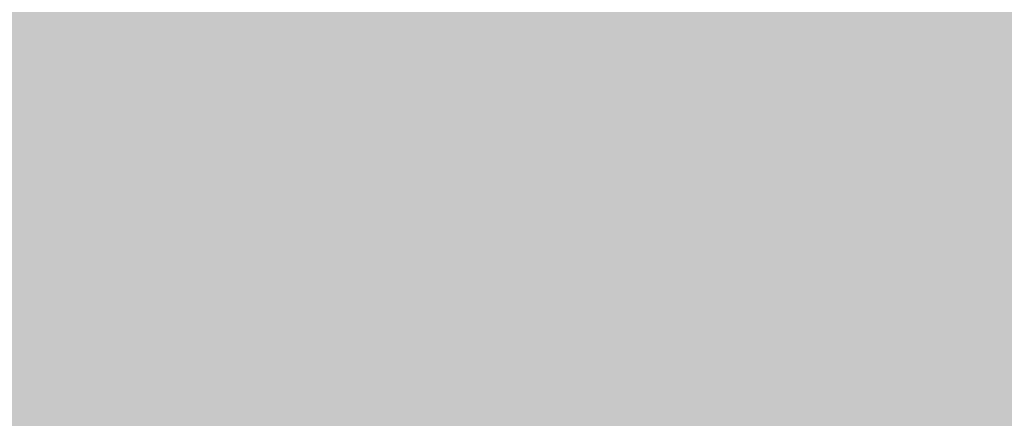
# Model space of a CAD drawing. Units: millimetres. Extents: x 0 to 2267, y 0 to 1823.
# Tile 102 of 256: x 1600.369 to 1605.705, y 1228.277 to 1230.439. Entities that reach past the tile are written whole.
import ezdxf

# ---------------------------------------------------------------- set-up
doc = ezdxf.new("R2010")
doc.units = ezdxf.units.MM
doc.header["$MEASUREMENT"] = 0
doc.layers.add('M-HATC', color=252, linetype='Continuous', lineweight=18)

msp = doc.modelspace()

# ---------------------------------------------------------------- hatches: boundary and pattern name
at = {"layer": 'M-HATC'}
h = msp.add_hatch(color=256, dxfattribs=at)
h.dxf.hatch_style = 1
h.paths.add_polyline_path([(2055.771, 1603.062), (1381.0868, 1603.062), (1381.0868, 1598.062), (2055.771, 1598.062)])
h.paths.add_polyline_path([(2055.771, 1598.062), (1381.0868, 1598.062), (1381.0868, 1593.062), (2055.771, 1593.062)])
h.paths.add_polyline_path([(2051.3074, 1536.7609), (1385.5504, 1536.7609), (1385.5504, 1526.7609), (1387.5504, 1526.7609), (1388.5366, 1525.0528), (1385.3319, 1521.2335), (1385.3319, 1521.2226), (2050.2542, 1522.7491), (2048.3212, 1525.0528), (2049.3074, 1526.7609), (2051.3074, 1526.7609)])
edge = h.paths.add_edge_path()
edge.add_arc((1847.5345, 1379.1492), 135, 222.603061, 222.890851, ccw=False)
edge.add_line((1748.1663, 1287.7656), (1683.0921, 1287.7656))
edge.add_arc((1583.7239, 1379.1492), 135, 317.109149, 317.396939, ccw=False)
edge.add_arc((1678.9686, 1290.6707), 5, 222.8909, 317.1091, ccw=False)
edge.add_arc((1774.2133, 1379.1492), 135, 222.603061, 222.890851, ccw=False)
edge.add_line((1674.8451, 1287.7656), (1609.7709, 1287.7656))
edge.add_arc((1510.4027, 1379.1492), 135, 317.109149, 317.396939, ccw=False)
edge.add_arc((1605.6474, 1290.6707), 5, 222.8909, 317.1091, ccw=False)
edge.add_arc((1700.8921, 1379.1492), 135, 222.603061, 222.890851, ccw=False)
edge.add_line((1601.5239, 1287.7656), (1536.4497, 1287.7656))
edge.add_arc((1437.0815, 1379.1492), 135, 317.109149, 317.396939, ccw=False)
edge.add_arc((1532.3262, 1290.6707), 5, 222.8909, 317.1091, ccw=False)
edge.add_arc((1627.5709, 1379.1492), 135, 222.603061, 222.890851, ccw=False)
edge.add_line((1528.2027, 1287.7656), (1505.9289, 1287.7656))
edge.add_spline(control_points=[(1505.9289, 1287.7656), (1504.2622, 1287.7656), (1504.2622, 1282.7656), (1505.9289, 1282.7656)], knot_values=[0, 0, 0, 0, 5, 5, 5, 5], degree=3, periodic=0)
edge.add_line((1505.9289, 1282.7656), (1930.9289, 1282.7656))
edge.add_spline(control_points=[(1930.9289, 1282.7656), (1932.5956, 1282.7656), (1932.5956, 1287.7656), (1930.9289, 1287.7656)], knot_values=[0, 0, 0, 0, 5, 5, 5, 5], degree=3, periodic=0)
edge.add_line((1930.9289, 1287.7656), (1903.0557, 1287.7656))
edge.add_arc((1803.6875, 1379.1492), 135, 317.109149, 317.396939, ccw=False)
edge.add_arc((1898.9322, 1290.6707), 5, 222.8909, 317.1091, ccw=False)
edge.add_arc((1994.1769, 1379.1492), 135, 222.603061, 222.890851, ccw=False)
edge.add_line((1894.8087, 1287.7656), (1829.7345, 1287.7656))
edge.add_arc((1730.3663, 1379.1492), 135, 317.109149, 317.396939, ccw=False)
edge.add_arc((1825.611, 1290.6707), 5, 222.8909, 317.1091, ccw=False)
edge.add_arc((1920.8557, 1379.1492), 135, 222.603061, 222.890851, ccw=False)
edge.add_line((1821.4875, 1287.7656), (1756.4133, 1287.7656))
edge.add_arc((1657.0451, 1379.1492), 135, 317.109149, 317.396939, ccw=False)
edge.add_arc((1752.2898, 1290.6707), 5, 222.8909, 317.1091, ccw=False)
edge = h.paths.add_edge_path()
edge.add_spline(control_points=[(1843.4289, 1227.2475), (1845.0956, 1227.2475), (1845.0956, 1232.2475), (1843.4289, 1232.2475)], knot_values=[0, 0, 0, 0, 5, 5, 5, 5], degree=3, periodic=0)
edge.add_line((1843.4289, 1232.2475), (1593.4289, 1232.2475))
edge.add_spline(control_points=[(1593.4289, 1232.2475), (1591.7622, 1232.2475), (1591.7622, 1227.2475), (1593.4289, 1227.2475)], knot_values=[0, 0, 0, 0, 5, 5, 5, 5], degree=3, periodic=0)
edge.add_line((1593.4289, 1227.2475), (1843.4289, 1227.2475))
h.paths.add_polyline_path([(1905.9289, 1127.4171), (1530.9289, 1127.4171, 0.414214), (1520.9289, 1117.4171), (1530.9289, 1117.4171), (1915.9289, 1117.4171, 0.414214)])
edge = h.paths.add_edge_path()
edge.add_arc((1397.0858, 1498.4078), 12.7299, 90.78215, 190.87871, ccw=False)
edge.add_line((1396.912, 1511.1365), (1428.0097, 1511.3488))
edge.add_line((1428.0097, 1511.3488), (1433.0097, 1511.3488))
edge.add_line((1433.0097, 1511.3488), (1434.439, 1511.3488))
edge.add_arc((1419.474, 1498.0804), 20, 41.561, 74.08211)
edge.add_line((1424.9592, 1517.3135), (1399.9351, 1517.2561))
edge.add_spline(control_points=[(1399.9307, 1517.2561), (1399.884, 1517.2131), (1399.8328, 1517.1689), (1399.7774, 1517.1236)], knot_values=[11.567499, 11.567499, 11.567499, 11.567499, 11.814249, 11.814249, 11.814249, 11.814249], degree=3, periodic=0)
edge.add_spline(control_points=[(1399.6328, 1517.0099), (1399.5831, 1516.9721), (1399.5307, 1516.9338), (1399.4759, 1516.8947)], knot_values=[11.167718, 11.167718, 11.167718, 11.167718, 11.365188, 11.365188, 11.365188, 11.365188], degree=3, periodic=0)
edge.add_spline(control_points=[(1399.3398, 1516.8001), (1399.1514, 1516.6719), (1398.9384, 1516.5377), (1398.704, 1516.3994)], knot_values=[10.376405, 10.376405, 10.376405, 10.376405, 11.00994, 11.00994, 11.00994, 11.00994], degree=3, periodic=0)
edge.add_spline(control_points=[(1398.6572, 1516.3719), (1398.5789, 1516.326), (1398.4983, 1516.2797), (1398.4155, 1516.2331)], knot_values=[10.125175, 10.125175, 10.125175, 10.125175, 10.334406, 10.334406, 10.334406, 10.334406], degree=3, periodic=0)
edge.add_spline(control_points=[(1398.2642, 1516.1487), (1398.196, 1516.1111), (1398.1263, 1516.0732), (1398.0555, 1516.0351)], knot_values=[9.832246, 9.832246, 9.832246, 9.832246, 9.999658, 9.999658, 9.999658, 9.999658], degree=3, periodic=0)
edge.add_spline(control_points=[(1397.9987, 1516.0048), (1397.7312, 1515.8621), (1397.446, 1515.7171), (1397.1466, 1515.5714)], knot_values=[9.161808, 9.161808, 9.161808, 9.161808, 9.787769, 9.787769, 9.787769, 9.787769], degree=3, periodic=0)
edge.add_spline(control_points=[(1397.1466, 1515.5714), (1396.8418, 1515.423), (1396.5222, 1515.274), (1396.1914, 1515.1262)], knot_values=[8.524455, 8.524455, 8.524455, 8.524455, 9.161808, 9.161808, 9.161808, 9.161808], degree=3, periodic=0)
edge.add_spline(control_points=[(1396.0777, 1515.0756), (1395.9854, 1515.0348), (1395.8922, 1514.994), (1395.7983, 1514.9534)], knot_values=[8.275193, 8.275193, 8.275193, 8.275193, 8.451726, 8.451726, 8.451726, 8.451726], degree=3, periodic=0)
edge.add_spline(control_points=[(1395.6018, 1514.8691), (1395.4997, 1514.8257), (1395.3968, 1514.7824), (1395.2932, 1514.7394)], knot_values=[7.962917, 7.962917, 7.962917, 7.962917, 8.152764, 8.152764, 8.152764, 8.152764], degree=3, periodic=0)
edge.add_spline(control_points=[(1395.2116, 1514.7057), (1394.8278, 1514.5475), (1394.4345, 1514.3929), (1394.0364, 1514.2442)], knot_values=[7.21254, 7.21254, 7.21254, 7.21254, 7.913148, 7.913148, 7.913148, 7.913148], degree=3, periodic=0)
edge.add_spline(control_points=[(1394.0364, 1514.2442), (1393.7076, 1514.1214), (1393.3754, 1514.0027), (1393.0427, 1513.8895)], knot_values=[6.633733, 6.633733, 6.633733, 6.633733, 7.21254, 7.21254, 7.21254, 7.21254], degree=3, periodic=0)
edge.add_spline(control_points=[(1392.8214, 1513.815), (1392.7198, 1513.7812), (1392.6181, 1513.7479), (1392.5166, 1513.7152)], knot_values=[6.328796, 6.328796, 6.328796, 6.328796, 6.505493, 6.505493, 6.505493, 6.505493], degree=3, periodic=0)
edge.add_spline(control_points=[(1392.5166, 1513.7152), (1392.3187, 1513.6515), (1392.1212, 1513.59), (1391.9244, 1513.531)], knot_values=[5.984605, 5.984605, 5.984605, 5.984605, 6.328796, 6.328796, 6.328796, 6.328796], degree=3, periodic=0)
edge.add_spline(control_points=[(1391.7915, 1513.4915), (1391.3122, 1513.3501), (1390.8384, 1513.2239), (1390.3784, 1513.1171)], knot_values=[5.066697, 5.066697, 5.066697, 5.066697, 5.907055, 5.907055, 5.907055, 5.907055], degree=3, periodic=0)
edge.add_spline(control_points=[(1390.3784, 1513.1171), (1390.1797, 1513.071), (1389.9836, 1513.0284), (1389.7907, 1512.9899)], knot_values=[4.70367, 4.70367, 4.70367, 4.70367, 5.066695, 5.066695, 5.066695, 5.066695], degree=3, periodic=0)
edge.add_spline(control_points=[(1389.422, 1512.9204), (1389.2459, 1512.8892), (1389.0729, 1512.8617), (1388.9036, 1512.8381)], knot_values=[4.130571, 4.130571, 4.130571, 4.130571, 4.469816, 4.469816, 4.469816, 4.469816], degree=3, periodic=0)
edge.add_spline(control_points=[(1388.9036, 1512.8381), (1388.591, 1512.7946), (1388.2911, 1512.7644), (1388.0071, 1512.7494)], knot_values=[3.504031, 3.504031, 3.504031, 3.504031, 4.130571, 4.130571, 4.130571, 4.130571], degree=3, periodic=0)
edge.add_spline(control_points=[(1387.9356, 1512.7459), (1387.8538, 1512.7423), (1387.7733, 1512.74), (1387.6944, 1512.739)], knot_values=[3.268866, 3.268866, 3.268866, 3.268866, 3.451164, 3.451164, 3.451164, 3.451164], degree=3, periodic=0)
edge.add_spline(control_points=[(1387.3351, 1512.7443), (1387.2076, 1512.7499), (1387.0847, 1512.7597), (1386.967, 1512.7739)], knot_values=[2.670686, 2.670686, 2.670686, 2.670686, 2.984, 2.984, 2.984, 2.984], degree=3, periodic=0)
edge.add_spline(control_points=[(1386.8327, 1512.7922), (1386.8209, 1512.7941), (1386.8092, 1512.7959), (1386.7975, 1512.7979)], knot_values=[2.516981, 2.516981, 2.516981, 2.516981, 2.549528, 2.549528, 2.549528, 2.549528], degree=3, periodic=0)
edge.add_spline(control_points=[(1386.4526, 1512.8735), (1386.4257, 1512.881), (1386.3993, 1512.889), (1386.3733, 1512.8972)], knot_values=[2.095869, 2.095869, 2.095869, 2.095869, 2.17941, 2.17941, 2.17941, 2.17941], degree=3, periodic=0)
edge.add_spline(control_points=[(1386.0691, 1513.0189), (1386.0634, 1513.0217), (1386.0577, 1513.0246), (1386.052, 1513.0275)], knot_values=[1.72453, 1.72453, 1.72453, 1.72453, 1.745933, 1.745933, 1.745933, 1.745933], degree=3, periodic=0)
edge.add_arc((1399.474, 1498.0804), 20, 131.82432, 180)
edge.add_arc((1630.3336, 1505.5484), 250.9708, 181.705176, 236.427975)
edge.add_arc((1605.3399, 1483.3044), 218.7822, 238.660829, 243.34961)
edge.add_arc((1647.0911, 1510.3592), 262.8986, 183.129836, 237.853442, ccw=False)
h.paths.add_polyline_path([(1406.5369, 1391.9644, 0.149382), (1491.5506, 1296.4418, -0.129517)], flags=17)
edge = h.paths.add_edge_path()
edge.add_arc((2037.3838, 1498.0804), 20, 0, 48.26587)
edge.add_spline(control_points=[(2050.6973, 1513.0052), (2050.6512, 1512.9847), (2050.6034, 1512.9655), (2050.5539, 1512.9477)], knot_values=[1.835652, 1.835652, 1.835652, 1.835652, 2.000781, 2.000781, 2.000781, 2.000781], degree=3, periodic=0)
edge.add_spline(control_points=[(2050.4616, 1512.9166), (2050.479, 1512.9221), (2050.4963, 1512.9277), (2050.5133, 1512.9335)], knot_values=[2.045477, 2.045477, 2.045477, 2.045477, 2.101389, 2.101389, 2.101389, 2.101389], degree=3, periodic=0)
edge.add_spline(control_points=[(2050.129, 1512.8342), (2050.1984, 1512.8473), (2050.2657, 1512.8623), (2050.3308, 1512.8792)], knot_values=[2.237629, 2.237629, 2.237629, 2.237629, 2.435841, 2.435841, 2.435841, 2.435841], degree=3, periodic=0)
edge.add_spline(control_points=[(2050.0946, 1512.8278), (2050.1061, 1512.8299), (2050.1176, 1512.832), (2050.129, 1512.8342)], knot_values=[2.435841, 2.435841, 2.435841, 2.435841, 2.468321, 2.468321, 2.468321, 2.468321], degree=3, periodic=0)
edge.add_spline(control_points=[(2049.7843, 1512.7851), (2049.8552, 1512.7922), (2049.9243, 1512.8008), (2049.9917, 1512.8109)], knot_values=[2.563852, 2.563852, 2.563852, 2.563852, 2.748541, 2.748541, 2.748541, 2.748541], degree=3, periodic=0)
edge.add_spline(control_points=[(2049.4052, 1512.7617), (2049.5364, 1512.7653), (2049.6629, 1512.773), (2049.7843, 1512.7851)], knot_values=[2.748541, 2.748541, 2.748541, 2.748541, 3.064882, 3.064882, 3.064882, 3.064882], degree=3, periodic=0)
edge.add_spline(control_points=[(2049.1698, 1512.7597), (2049.2336, 1512.7591), (2049.2965, 1512.7594), (2049.3584, 1512.7606)], knot_values=[3.102309, 3.102309, 3.102309, 3.102309, 3.2503, 3.2503, 3.2503, 3.2503], degree=3, periodic=0)
edge.add_spline(control_points=[(2048.8573, 1512.7691), (2048.9638, 1512.7638), (2049.068, 1512.7606), (2049.1698, 1512.7597)], knot_values=[3.2503, 3.2503, 3.2503, 3.2503, 3.486069, 3.486069, 3.486069, 3.486069], degree=3, periodic=0)
edge.add_spline(control_points=[(2048.6924, 1512.7789), (2048.3729, 1512.8009), (2048.0345, 1512.8411), (2047.6817, 1512.897)], knot_values=[3.606429, 3.606429, 3.606429, 3.606429, 4.2989, 4.2989, 4.2989, 4.2989], degree=3, periodic=0)
edge.add_spline(control_points=[(2047.6817, 1512.897), (2047.5458, 1512.9185), (2047.4077, 1512.9424), (2047.2678, 1512.9685)], knot_values=[4.2989, 4.2989, 4.2989, 4.2989, 4.565769, 4.565769, 4.565769, 4.565769], degree=3, periodic=0)
edge.add_spline(control_points=[(2047.2678, 1512.9685), (2047.1449, 1512.9914), (2047.0207, 1513.016), (2046.8951, 1513.0422)], knot_values=[4.565769, 4.565769, 4.565769, 4.565769, 4.799971, 4.799971, 4.799971, 4.799971], degree=3, periodic=0)
edge.add_spline(control_points=[(2046.8951, 1513.0422), (2046.5286, 1513.1188), (2046.1513, 1513.209), (2045.7676, 1513.3107)], knot_values=[4.799971, 4.799971, 4.799971, 4.799971, 5.483718, 5.483718, 5.483718, 5.483718], degree=3, periodic=0)
edge.add_spline(control_points=[(2045.7676, 1513.3107), (2045.3724, 1513.4154), (2044.9704, 1513.5322), (2044.5662, 1513.6588)], knot_values=[5.483718, 5.483718, 5.483718, 5.483718, 6.187866, 6.187866, 6.187866, 6.187866], degree=3, periodic=0)
edge.add_spline(control_points=[(2044.5662, 1513.6588), (2044.4149, 1513.7061), (2044.2633, 1513.7549), (2044.1116, 1513.8048)], knot_values=[6.187866, 6.187866, 6.187866, 6.187866, 6.451551, 6.451551, 6.451551, 6.451551], degree=3, periodic=0)
edge.add_spline(control_points=[(2044.1116, 1513.8048), (2043.9967, 1513.8427), (2043.8817, 1513.8813), (2043.7668, 1513.9205)], knot_values=[6.451551, 6.451551, 6.451551, 6.451551, 6.651434, 6.651434, 6.651434, 6.651434], degree=3, periodic=0)
edge.add_spline(control_points=[(2043.7668, 1513.9205), (2043.3716, 1514.0554), (2042.9774, 1514.1979), (2042.5886, 1514.3458)], knot_values=[6.651434, 6.651434, 6.651434, 6.651434, 7.338879, 7.338879, 7.338879, 7.338879], degree=3, periodic=0)
edge.add_spline(control_points=[(2042.5886, 1514.3458), (2042.1643, 1514.5071), (2041.7465, 1514.6749), (2041.3409, 1514.846)], knot_values=[7.338879, 7.338879, 7.338879, 7.338879, 8.089209, 8.089209, 8.089209, 8.089209], degree=3, periodic=0)
edge.add_spline(control_points=[(2041.3409, 1514.846), (2041.1028, 1514.9465), (2040.869, 1515.0481), (2040.6405, 1515.1502)], knot_values=[8.089209, 8.089209, 8.089209, 8.089209, 8.529587, 8.529587, 8.529587, 8.529587], degree=3, periodic=0)
edge.add_spline(control_points=[(2040.51, 1515.2089), (2040.0824, 1515.4022), (2039.6747, 1515.5971), (2039.295, 1515.7894)], knot_values=[8.613818, 8.613818, 8.613818, 8.613818, 9.44571, 9.44571, 9.44571, 9.44571], degree=3, periodic=0)
edge.add_spline(control_points=[(2039.295, 1515.7894), (2039.0618, 1515.9075), (2038.8391, 1516.0246), (2038.6288, 1516.1398)], knot_values=[9.44571, 9.44571, 9.44571, 9.44571, 9.956404, 9.956404, 9.956404, 9.956404], degree=3, periodic=0)
edge.add_spline(control_points=[(2038.6288, 1516.1398), (2038.5187, 1516.2001), (2038.4121, 1516.2598), (2038.309, 1516.3189)], knot_values=[9.956404, 9.956404, 9.956404, 9.956404, 10.223542, 10.223542, 10.223542, 10.223542], degree=3, periodic=0)
edge.add_spline(control_points=[(2038.309, 1516.3189), (2038.2138, 1516.3735), (2038.1216, 1516.4276), (2038.0328, 1516.481)], knot_values=[10.223542, 10.223542, 10.223542, 10.223542, 10.47051, 10.47051, 10.47051, 10.47051], degree=3, periodic=0)
edge.add_spline(control_points=[(2038.0328, 1516.481), (2037.7855, 1516.6296), (2037.5639, 1516.773), (2037.3722, 1516.909)], knot_values=[10.47051, 10.47051, 10.47051, 10.47051, 11.15767, 11.15767, 11.15767, 11.15767], degree=3, periodic=0)
edge.add_spline(control_points=[(2037.3722, 1516.909), (2037.2789, 1516.9752), (2037.1927, 1517.0396), (2037.1142, 1517.102)], knot_values=[11.15767, 11.15767, 11.15767, 11.15767, 11.49227, 11.49227, 11.49227, 11.49227], degree=3, periodic=0)
edge.add_spline(control_points=[(2036.8564, 1517.3259), (2036.9148, 1517.2692), (2036.9814, 1517.2103), (2037.0557, 1517.1492)], knot_values=[11.577341, 11.577341, 11.577341, 11.577341, 11.91035, 11.91035, 11.91035, 11.91035], degree=3, periodic=0)
edge.add_spline(control_points=[(2036.8074, 1517.3748), (2036.823, 1517.3587), (2036.8393, 1517.3424), (2036.8564, 1517.3259)], knot_values=[11.91035, 11.91035, 11.91035, 11.91035, 12.007402, 12.007402, 12.007402, 12.007402], degree=3, periodic=0)
edge.add_spline(control_points=[(2036.7017, 1517.494), (2036.7104, 1517.483), (2036.7196, 1517.4719), (2036.7291, 1517.4606)], knot_values=[12.184155, 12.184155, 12.184155, 12.184155, 12.255409, 12.255409, 12.255409, 12.255409], degree=3, periodic=0)
edge.add_spline(control_points=[(2036.6159, 1517.6205), (2036.62, 1517.613), (2036.6243, 1517.6055), (2036.6289, 1517.5979)], knot_values=[12.487913, 12.487913, 12.487913, 12.487913, 12.541035, 12.541035, 12.541035, 12.541035], degree=3, periodic=0)
edge.add_spline(control_points=[(2036.5635, 1517.786), (2036.5637, 1517.7794), (2036.5642, 1517.7726), (2036.565, 1517.7658)], knot_values=[12.911761, 12.911761, 12.911761, 12.911761, 12.968286, 12.968286, 12.968286, 12.968286], degree=3, periodic=0)
edge.add_spline(control_points=[(2036.6166, 1517.9304), (2036.6125, 1517.9259), (2036.6086, 1517.9212), (2036.6049, 1517.9165)], knot_values=[13.382527, 13.382527, 13.382527, 13.382527, 13.433791, 13.433791, 13.433791, 13.433791], degree=3, periodic=0)
edge.add_spline(control_points=[(2036.749, 1518.017), (2036.7361, 1518.0116), (2036.7239, 1518.006), (2036.7124, 1518.0002)], knot_values=[13.726299, 13.726299, 13.726299, 13.726299, 13.809928, 13.809928, 13.809928, 13.809928], degree=3, periodic=0)
edge.add_spline(control_points=[(2036.8604, 1518.0528), (2036.8386, 1518.0474), (2036.8181, 1518.0416), (2036.7988, 1518.0353)], knot_values=[13.910887, 13.910887, 13.910887, 13.910887, 14.02153, 14.02153, 14.02153, 14.02153], degree=3, periodic=0)
edge.add_line((2036.9639, 1518.0804), (2032.3838, 1518.0804))
edge.add_line((2032.3838, 1518.0804), (2027.3838, 1518.0804))
edge.add_line((2027.3838, 1518.0804), (2022.3838, 1518.0804))
edge.add_line((2022.3838, 1518.0804), (2017.3838, 1518.0804))
edge.add_arc((2017.3838, 1498.0804), 20, 90, 138.439)
edge.add_line((2002.4188, 1511.3488), (2003.8481, 1511.3488))
edge.add_line((2003.8481, 1511.3488), (2008.8481, 1511.3488))
edge.add_line((2008.8481, 1511.3488), (2039.772, 1511.1377))
edge.add_arc((2039.772, 1498.4078), 12.7299, -10.87871, 90, ccw=False)
edge.add_arc((1789.7668, 1510.3592), 262.8986, 302.146558, 356.870164, ccw=False)
edge.add_arc((1831.5179, 1483.3044), 218.7822, 296.65039, 301.339171)
edge.add_arc((1806.5242, 1505.5484), 250.9708, 303.572025, 358.294824)
h.paths.add_polyline_path([(2030.321, 1391.9644, -0.129517), (1945.3072, 1296.4418, 0.149382)], flags=17)
edge = h.paths.add_edge_path()
edge.add_spline(control_points=[(2037.2464, 1518.0821), (2037.2898, 1518.081), (2037.3355, 1518.0804), (2037.3838, 1518.0804)], knot_values=[0.000012, 0.000012, 0.000012, 0.000012, 0.144754, 0.144754, 0.144754, 0.144754], degree=3, periodic=0)
edge.add_line((2037.3357, 1518.0804), (2037.0096, 1518.0804))
edge.add_spline(control_points=[(2037.0096, 1518.0804), (2036.9822, 1518.0768), (2036.956, 1518.0727), (2036.9312, 1518.0681)], knot_values=[14.13465, 14.13465, 14.13465, 14.13465, 14.247197, 14.247197, 14.247197, 14.247197], degree=3, periodic=0)
edge.add_spline(control_points=[(2036.9312, 1518.0681), (2036.9276, 1518.0674), (2036.9241, 1518.0667), (2036.9205, 1518.0661)], knot_values=[14.118315, 14.118315, 14.118315, 14.118315, 14.13465, 14.13465, 14.13465, 14.13465], degree=3, periodic=0)
edge.add_spline(control_points=[(2036.9205, 1518.0661), (2036.9118, 1518.0644), (2036.9032, 1518.0626), (2036.8948, 1518.0608)], knot_values=[14.078086, 14.078086, 14.078086, 14.078086, 14.118315, 14.118315, 14.118315, 14.118315], degree=3, periodic=0)
edge.add_spline(control_points=[(2036.8948, 1518.0608), (2036.883, 1518.0583), (2036.8716, 1518.0556), (2036.8604, 1518.0528)], knot_values=[14.02153, 14.02153, 14.02153, 14.02153, 14.078086, 14.078086, 14.078086, 14.078086], degree=3, periodic=0)
edge.add_spline(control_points=[(2036.8604, 1518.0528), (2036.8386, 1518.0474), (2036.8181, 1518.0416), (2036.7988, 1518.0353)], knot_values=[13.910887, 13.910887, 13.910887, 13.910887, 14.02153, 14.02153, 14.02153, 14.02153], degree=3, periodic=0)
edge.add_spline(control_points=[(2036.7988, 1518.0353), (2036.7981, 1518.035), (2036.7974, 1518.0348), (2036.7967, 1518.0346)], knot_values=[13.906906, 13.906906, 13.906906, 13.906906, 13.910887, 13.910887, 13.910887, 13.910887], degree=3, periodic=0)
edge.add_spline(control_points=[(2036.7967, 1518.0346), (2036.7882, 1518.0318), (2036.7799, 1518.0289), (2036.7719, 1518.0259)], knot_values=[13.857826, 13.857826, 13.857826, 13.857826, 13.906906, 13.906906, 13.906906, 13.906906], degree=3, periodic=0)
edge.add_spline(control_points=[(2036.7719, 1518.0259), (2036.764, 1518.023), (2036.7564, 1518.02), (2036.749, 1518.017)], knot_values=[13.809928, 13.809928, 13.809928, 13.809928, 13.857826, 13.857826, 13.857826, 13.857826], degree=3, periodic=0)
edge.add_spline(control_points=[(2036.749, 1518.017), (2036.7361, 1518.0116), (2036.7239, 1518.006), (2036.7124, 1518.0002)], knot_values=[13.726299, 13.726299, 13.726299, 13.726299, 13.809928, 13.809928, 13.809928, 13.809928], degree=3, periodic=0)
edge.add_spline(control_points=[(2036.7124, 1518.0002), (2036.7121, 1518), (2036.7118, 1517.9999), (2036.7115, 1517.9997)], knot_values=[13.723993, 13.723993, 13.723993, 13.723993, 13.726299, 13.726299, 13.726299, 13.726299], degree=3, periodic=0)
edge.add_spline(control_points=[(2036.7115, 1517.9997), (2036.7063, 1517.9971), (2036.7013, 1517.9944), (2036.6965, 1517.9917)], knot_values=[13.686536, 13.686536, 13.686536, 13.686536, 13.723993, 13.723993, 13.723993, 13.723993], degree=3, periodic=0)
edge.add_spline(control_points=[(2036.6965, 1517.9917), (2036.6919, 1517.9891), (2036.6874, 1517.9865), (2036.6831, 1517.9839)], knot_values=[13.651251, 13.651251, 13.651251, 13.651251, 13.686536, 13.686536, 13.686536, 13.686536], degree=3, periodic=0)
edge.add_spline(control_points=[(2036.6831, 1517.9839), (2036.6764, 1517.9798), (2036.67, 1517.9757), (2036.6639, 1517.9714)], knot_values=[13.596804, 13.596804, 13.596804, 13.596804, 13.651251, 13.651251, 13.651251, 13.651251], degree=3, periodic=0)
edge.add_spline(control_points=[(2036.6639, 1517.9714), (2036.6636, 1517.9712), (2036.6633, 1517.9709), (2036.6629, 1517.9707)], knot_values=[13.593956, 13.593956, 13.593956, 13.593956, 13.596804, 13.596804, 13.596804, 13.596804], degree=3, periodic=0)
edge.add_spline(control_points=[(2036.6629, 1517.9707), (2036.6603, 1517.9689), (2036.6577, 1517.967), (2036.6552, 1517.9651)], knot_values=[13.570322, 13.570322, 13.570322, 13.570322, 13.593956, 13.593956, 13.593956, 13.593956], degree=3, periodic=0)
edge.add_spline(control_points=[(2036.6552, 1517.9651), (2036.6525, 1517.9631), (2036.6499, 1517.9611), (2036.6474, 1517.9591)], knot_values=[13.545477, 13.545477, 13.545477, 13.545477, 13.570322, 13.570322, 13.570322, 13.570322], degree=3, periodic=0)
edge.add_spline(control_points=[(2036.6474, 1517.9591), (2036.6472, 1517.9589), (2036.6471, 1517.9588), (2036.6469, 1517.9587)], knot_values=[13.543931, 13.543931, 13.543931, 13.543931, 13.545477, 13.545477, 13.545477, 13.545477], degree=3, periodic=0)
edge.add_spline(control_points=[(2036.6469, 1517.9587), (2036.6412, 1517.9541), (2036.6358, 1517.9494), (2036.6307, 1517.9447)], knot_values=[13.488237, 13.488237, 13.488237, 13.488237, 13.543931, 13.543931, 13.543931, 13.543931], degree=3, periodic=0)
edge.add_spline(control_points=[(2036.6307, 1517.9447), (2036.6282, 1517.9423), (2036.6257, 1517.9399), (2036.6233, 1517.9374)], knot_values=[13.460307, 13.460307, 13.460307, 13.460307, 13.488237, 13.488237, 13.488237, 13.488237], degree=3, periodic=0)
edge.add_spline(control_points=[(2036.6233, 1517.9374), (2036.6215, 1517.9356), (2036.6198, 1517.9338), (2036.6181, 1517.932)], knot_values=[13.439712, 13.439712, 13.439712, 13.439712, 13.460307, 13.460307, 13.460307, 13.460307], degree=3, periodic=0)
edge.add_spline(control_points=[(2036.6181, 1517.932), (2036.6176, 1517.9315), (2036.6171, 1517.9309), (2036.6166, 1517.9304)], knot_values=[13.433791, 13.433791, 13.433791, 13.433791, 13.439712, 13.439712, 13.439712, 13.439712], degree=3, periodic=0)
edge.add_spline(control_points=[(2036.6166, 1517.9304), (2036.6125, 1517.9259), (2036.6086, 1517.9212), (2036.6049, 1517.9165)], knot_values=[13.382527, 13.382527, 13.382527, 13.382527, 13.433791, 13.433791, 13.433791, 13.433791], degree=3, periodic=0)
edge.add_spline(control_points=[(2036.6049, 1517.9165), (2036.6026, 1517.9135), (2036.6004, 1517.9104), (2036.5982, 1517.9074)], knot_values=[13.350017, 13.350017, 13.350017, 13.350017, 13.382527, 13.382527, 13.382527, 13.382527], degree=3, periodic=0)
edge.add_spline(control_points=[(2036.5982, 1517.9074), (2036.5972, 1517.9059), (2036.5962, 1517.9043), (2036.5952, 1517.9028)], knot_values=[13.333922, 13.333922, 13.333922, 13.333922, 13.350017, 13.350017, 13.350017, 13.350017], degree=3, periodic=0)
edge.add_spline(control_points=[(2036.5952, 1517.9028), (2036.5945, 1517.9018), (2036.5939, 1517.9009), (2036.5933, 1517.8999)], knot_values=[13.323828, 13.323828, 13.323828, 13.323828, 13.333922, 13.333922, 13.333922, 13.333922], degree=3, periodic=0)
edge.add_spline(control_points=[(2036.5933, 1517.8999), (2036.5905, 1517.8955), (2036.5879, 1517.8909), (2036.5855, 1517.8864)], knot_values=[13.277545, 13.277545, 13.277545, 13.277545, 13.323828, 13.323828, 13.323828, 13.323828], degree=3, periodic=0)
edge.add_spline(control_points=[(2036.5855, 1517.8864), (2036.5836, 1517.8827), (2036.5817, 1517.8789), (2036.5801, 1517.8751)], knot_values=[13.240119, 13.240119, 13.240119, 13.240119, 13.277545, 13.277545, 13.277545, 13.277545], degree=3, periodic=0)
edge.add_spline(control_points=[(2036.5801, 1517.8751), (2036.5795, 1517.8739), (2036.579, 1517.8727), (2036.5785, 1517.8715)], knot_values=[13.228211, 13.228211, 13.228211, 13.228211, 13.240119, 13.240119, 13.240119, 13.240119], degree=3, periodic=0)
edge.add_spline(control_points=[(2036.5785, 1517.8715), (2036.578, 1517.8702), (2036.5774, 1517.869), (2036.5769, 1517.8677)], knot_values=[13.215717, 13.215717, 13.215717, 13.215717, 13.228211, 13.228211, 13.228211, 13.228211], degree=3, periodic=0)
edge.add_spline(control_points=[(2036.5769, 1517.8677), (2036.5755, 1517.864), (2036.5741, 1517.8603), (2036.5729, 1517.8565)], knot_values=[13.179847, 13.179847, 13.179847, 13.179847, 13.215717, 13.215717, 13.215717, 13.215717], degree=3, periodic=0)
edge.add_spline(control_points=[(2036.5729, 1517.8565), (2036.5713, 1517.8515), (2036.5699, 1517.8464), (2036.5687, 1517.8413)], knot_values=[13.132017, 13.132017, 13.132017, 13.132017, 13.179847, 13.179847, 13.179847, 13.179847], degree=3, periodic=0)
edge.add_spline(control_points=[(2036.5687, 1517.8413), (2036.5684, 1517.8402), (2036.5682, 1517.8392), (2036.568, 1517.8382)], knot_values=[13.122482, 13.122482, 13.122482, 13.122482, 13.132017, 13.132017, 13.132017, 13.132017], degree=3, periodic=0)
edge.add_spline(control_points=[(2036.568, 1517.8382), (2036.5676, 1517.8363), (2036.5672, 1517.8345), (2036.5669, 1517.8327)], knot_values=[13.105592, 13.105592, 13.105592, 13.105592, 13.122482, 13.122482, 13.122482, 13.122482], degree=3, periodic=0)
edge.add_spline(control_points=[(2036.5669, 1517.8327), (2036.5662, 1517.8292), (2036.5657, 1517.8257), (2036.5652, 1517.8222)], knot_values=[13.074063, 13.074063, 13.074063, 13.074063, 13.105592, 13.105592, 13.105592, 13.105592], degree=3, periodic=0)
edge.add_spline(control_points=[(2036.5652, 1517.8222), (2036.5652, 1517.8222), (2036.5652, 1517.8222), (2036.5652, 1517.8222)], knot_values=[13.074043, 13.074043, 13.074043, 13.074043, 13.074063, 13.074063, 13.074063, 13.074063], degree=3, periodic=0)
edge.add_spline(control_points=[(2036.5652, 1517.8222), (2036.5644, 1517.8164), (2036.5639, 1517.8106), (2036.5636, 1517.8046)], knot_values=[13.021884, 13.021884, 13.021884, 13.021884, 13.074043, 13.074043, 13.074043, 13.074043], degree=3, periodic=0)
edge.add_spline(control_points=[(2036.5636, 1517.8046), (2036.5636, 1517.804), (2036.5636, 1517.8034), (2036.5635, 1517.8028)], knot_values=[13.01674, 13.01674, 13.01674, 13.01674, 13.021884, 13.021884, 13.021884, 13.021884], degree=3, periodic=0)
edge.add_spline(control_points=[(2036.5635, 1517.8028), (2036.5634, 1517.8005), (2036.5634, 1517.7982), (2036.5634, 1517.7958)], knot_values=[12.996438, 12.996438, 12.996438, 12.996438, 13.01674, 13.01674, 13.01674, 13.01674], degree=3, periodic=0)
edge.add_spline(control_points=[(2036.5634, 1517.7958), (2036.5633, 1517.7926), (2036.5634, 1517.7893), (2036.5635, 1517.786)], knot_values=[12.968286, 12.968286, 12.968286, 12.968286, 12.996438, 12.996438, 12.996438, 12.996438], degree=3, periodic=0)
edge.add_spline(control_points=[(2036.5635, 1517.786), (2036.5637, 1517.7794), (2036.5642, 1517.7726), (2036.565, 1517.7658)], knot_values=[12.911761, 12.911761, 12.911761, 12.911761, 12.968286, 12.968286, 12.968286, 12.968286], degree=3, periodic=0)
edge.add_spline(control_points=[(2036.565, 1517.7658), (2036.565, 1517.7657), (2036.565, 1517.7656), (2036.565, 1517.7656)], knot_values=[12.911017, 12.911017, 12.911017, 12.911017, 12.911761, 12.911761, 12.911761, 12.911761], degree=3, periodic=0)
edge.add_spline(control_points=[(2036.565, 1517.7656), (2036.5654, 1517.7625), (2036.5658, 1517.7593), (2036.5663, 1517.7562)], knot_values=[12.88528, 12.88528, 12.88528, 12.88528, 12.911017, 12.911017, 12.911017, 12.911017], degree=3, periodic=0)
edge.add_spline(control_points=[(2036.5663, 1517.7562), (2036.5667, 1517.7534), (2036.5672, 1517.7506), (2036.5677, 1517.7478)], knot_values=[12.862519, 12.862519, 12.862519, 12.862519, 12.88528, 12.88528, 12.88528, 12.88528], degree=3, periodic=0)
edge.add_spline(control_points=[(2036.5677, 1517.7478), (2036.5678, 1517.7474), (2036.5679, 1517.7469), (2036.568, 1517.7465)], knot_values=[12.858885, 12.858885, 12.858885, 12.858885, 12.862519, 12.862519, 12.862519, 12.862519], degree=3, periodic=0)
edge.add_spline(control_points=[(2036.568, 1517.7465), (2036.5692, 1517.7399), (2036.5707, 1517.7332), (2036.5724, 1517.7264)], knot_values=[12.8053, 12.8053, 12.8053, 12.8053, 12.858885, 12.858885, 12.858885, 12.858885], degree=3, periodic=0)
edge.add_spline(control_points=[(2036.5724, 1517.7264), (2036.5734, 1517.7226), (2036.5745, 1517.7187), (2036.5756, 1517.7149)], knot_values=[12.775176, 12.775176, 12.775176, 12.775176, 12.8053, 12.8053, 12.8053, 12.8053], degree=3, periodic=0)
edge.add_spline(control_points=[(2036.5756, 1517.7149), (2036.5763, 1517.7125), (2036.577, 1517.7102), (2036.5778, 1517.7078)], knot_values=[12.756759, 12.756759, 12.756759, 12.756759, 12.775176, 12.775176, 12.775176, 12.775176], degree=3, periodic=0)
edge.add_spline(control_points=[(2036.5778, 1517.7078), (2036.5781, 1517.7067), (2036.5784, 1517.7057), (2036.5787, 1517.7047)], knot_values=[12.748742, 12.748742, 12.748742, 12.748742, 12.756759, 12.756759, 12.756759, 12.756759], degree=3, periodic=0)
edge.add_spline(control_points=[(2036.5787, 1517.7047), (2036.5808, 1517.6983), (2036.5831, 1517.6919), (2036.5856, 1517.6854)], knot_values=[12.69959, 12.69959, 12.69959, 12.69959, 12.748742, 12.748742, 12.748742, 12.748742], degree=3, periodic=0)
edge.add_spline(control_points=[(2036.5856, 1517.6854), (2036.5876, 1517.68), (2036.5898, 1517.6746), (2036.5921, 1517.6692)], knot_values=[12.659038, 12.659038, 12.659038, 12.659038, 12.69959, 12.69959, 12.69959, 12.69959], degree=3, periodic=0)
edge.add_spline(control_points=[(2036.5921, 1517.6692), (2036.594, 1517.6648), (2036.5959, 1517.6605), (2036.5979, 1517.6561)], knot_values=[12.626806, 12.626806, 12.626806, 12.626806, 12.659038, 12.659038, 12.659038, 12.659038], degree=3, periodic=0)
edge.add_spline(control_points=[(2036.5979, 1517.6561), (2036.5984, 1517.6551), (2036.5989, 1517.6541), (2036.5993, 1517.6531)], knot_values=[12.619394, 12.619394, 12.619394, 12.619394, 12.626806, 12.626806, 12.626806, 12.626806], degree=3, periodic=0)
edge.add_spline(control_points=[(2036.5993, 1517.6531), (2036.6043, 1517.6424), (2036.6099, 1517.6315), (2036.6159, 1517.6205)], knot_values=[12.541039, 12.541039, 12.541039, 12.541039, 12.619394, 12.619394, 12.619394, 12.619394], degree=3, periodic=0)
edge.add_spline(control_points=[(2036.6159, 1517.6205), (2036.6159, 1517.6205), (2036.6159, 1517.6205), (2036.6159, 1517.6205)], knot_values=[12.541035, 12.541035, 12.541035, 12.541035, 12.541039, 12.541039, 12.541039, 12.541039], degree=3, periodic=0)
edge.add_spline(control_points=[(2036.6159, 1517.6205), (2036.62, 1517.613), (2036.6243, 1517.6055), (2036.6289, 1517.5979)], knot_values=[12.487913, 12.487913, 12.487913, 12.487913, 12.541035, 12.541035, 12.541035, 12.541035], degree=3, periodic=0)
edge.add_spline(control_points=[(2036.6289, 1517.5979), (2036.6326, 1517.5916), (2036.6365, 1517.5853), (2036.6406, 1517.5789)], knot_values=[12.443982, 12.443982, 12.443982, 12.443982, 12.487913, 12.487913, 12.487913, 12.487913], degree=3, periodic=0)
edge.add_spline(control_points=[(2036.6406, 1517.5789), (2036.6414, 1517.5776), (2036.6423, 1517.5763), (2036.6431, 1517.5749)], knot_values=[12.434996, 12.434996, 12.434996, 12.434996, 12.443982, 12.443982, 12.443982, 12.443982], degree=3, periodic=0)
edge.add_spline(control_points=[(2036.6431, 1517.5749), (2036.6531, 1517.5596), (2036.6639, 1517.5439), (2036.6756, 1517.528)], knot_values=[12.329647, 12.329647, 12.329647, 12.329647, 12.434996, 12.434996, 12.434996, 12.434996], degree=3, periodic=0)
edge.add_spline(control_points=[(2036.6756, 1517.528), (2036.6839, 1517.5168), (2036.6925, 1517.5055), (2036.7017, 1517.494)], knot_values=[12.255409, 12.255409, 12.255409, 12.255409, 12.329647, 12.329647, 12.329647, 12.329647], degree=3, periodic=0)
edge.add_spline(control_points=[(2036.7017, 1517.494), (2036.7104, 1517.483), (2036.7196, 1517.4719), (2036.7291, 1517.4606)], knot_values=[12.184155, 12.184155, 12.184155, 12.184155, 12.255409, 12.255409, 12.255409, 12.255409], degree=3, periodic=0)
edge.add_spline(control_points=[(2036.7291, 1517.4606), (2036.7436, 1517.4435), (2036.759, 1517.4262), (2036.7753, 1517.4085)], knot_values=[12.075961, 12.075961, 12.075961, 12.075961, 12.184155, 12.184155, 12.184155, 12.184155], degree=3, periodic=0)
edge.add_spline(control_points=[(2036.7753, 1517.4085), (2036.7763, 1517.4075), (2036.7773, 1517.4064), (2036.7783, 1517.4054)], knot_values=[12.069502, 12.069502, 12.069502, 12.069502, 12.075961, 12.075961, 12.075961, 12.075961], degree=3, periodic=0)
edge.add_spline(control_points=[(2036.7783, 1517.4054), (2036.7877, 1517.3953), (2036.7974, 1517.385), (2036.8074, 1517.3748)], knot_values=[12.007402, 12.007402, 12.007402, 12.007402, 12.069502, 12.069502, 12.069502, 12.069502], degree=3, periodic=0)
edge.add_spline(control_points=[(2036.8074, 1517.3748), (2036.823, 1517.3587), (2036.8393, 1517.3424), (2036.8564, 1517.3259)], knot_values=[11.91035, 11.91035, 11.91035, 11.91035, 12.007402, 12.007402, 12.007402, 12.007402], degree=3, periodic=0)
edge.add_spline(control_points=[(2036.8564, 1517.3259), (2036.9148, 1517.2692), (2036.9814, 1517.2103), (2037.0557, 1517.1492)], knot_values=[11.577341, 11.577341, 11.577341, 11.577341, 11.91035, 11.91035, 11.91035, 11.91035], degree=3, periodic=0)
edge.add_spline(control_points=[(2037.0557, 1517.1492), (2037.0747, 1517.1336), (2037.0942, 1517.1179), (2037.1142, 1517.102)], knot_values=[11.49227, 11.49227, 11.49227, 11.49227, 11.577341, 11.577341, 11.577341, 11.577341], degree=3, periodic=0)
edge.add_spline(control_points=[(2037.1142, 1517.102), (2037.1927, 1517.0396), (2037.2789, 1516.9752), (2037.3722, 1516.909)], knot_values=[11.15767, 11.15767, 11.15767, 11.15767, 11.49227, 11.49227, 11.49227, 11.49227], degree=3, periodic=0)
edge.add_spline(control_points=[(2037.3722, 1516.909), (2037.5639, 1516.773), (2037.7855, 1516.6296), (2038.0328, 1516.481)], knot_values=[10.47051, 10.47051, 10.47051, 10.47051, 11.15767, 11.15767, 11.15767, 11.15767], degree=3, periodic=0)
edge.add_spline(control_points=[(2038.0328, 1516.481), (2038.1216, 1516.4276), (2038.2138, 1516.3735), (2038.309, 1516.3189)], knot_values=[10.223542, 10.223542, 10.223542, 10.223542, 10.47051, 10.47051, 10.47051, 10.47051], degree=3, periodic=0)
edge.add_spline(control_points=[(2038.309, 1516.3189), (2038.4121, 1516.2598), (2038.5187, 1516.2001), (2038.6288, 1516.1398)], knot_values=[9.956404, 9.956404, 9.956404, 9.956404, 10.223542, 10.223542, 10.223542, 10.223542], degree=3, periodic=0)
edge.add_spline(control_points=[(2038.6288, 1516.1398), (2038.8391, 1516.0246), (2039.0618, 1515.9075), (2039.295, 1515.7894)], knot_values=[9.44571, 9.44571, 9.44571, 9.44571, 9.956404, 9.956404, 9.956404, 9.956404], degree=3, periodic=0)
edge.add_spline(control_points=[(2039.295, 1515.7894), (2039.6747, 1515.5971), (2040.0824, 1515.4022), (2040.51, 1515.2089)], knot_values=[8.613818, 8.613818, 8.613818, 8.613818, 9.44571, 9.44571, 9.44571, 9.44571], degree=3, periodic=0)
edge.add_spline(control_points=[(2040.51, 1515.2089), (2040.5533, 1515.1893), (2040.5968, 1515.1697), (2040.6405, 1515.1502)], knot_values=[8.529587, 8.529587, 8.529587, 8.529587, 8.613818, 8.613818, 8.613818, 8.613818], degree=3, periodic=0)
edge.add_spline(control_points=[(2040.6405, 1515.1502), (2040.869, 1515.0481), (2041.1028, 1514.9465), (2041.3409, 1514.846)], knot_values=[8.089209, 8.089209, 8.089209, 8.089209, 8.529587, 8.529587, 8.529587, 8.529587], degree=3, periodic=0)
edge.add_spline(control_points=[(2041.3409, 1514.846), (2041.7465, 1514.6749), (2042.1643, 1514.5071), (2042.5886, 1514.3458)], knot_values=[7.338879, 7.338879, 7.338879, 7.338879, 8.089209, 8.089209, 8.089209, 8.089209], degree=3, periodic=0)
edge.add_spline(control_points=[(2042.5886, 1514.3458), (2042.9774, 1514.1979), (2043.3716, 1514.0554), (2043.7668, 1513.9205)], knot_values=[6.651434, 6.651434, 6.651434, 6.651434, 7.338879, 7.338879, 7.338879, 7.338879], degree=3, periodic=0)
edge.add_spline(control_points=[(2043.7668, 1513.9205), (2043.8817, 1513.8813), (2043.9967, 1513.8427), (2044.1116, 1513.8048)], knot_values=[6.451551, 6.451551, 6.451551, 6.451551, 6.651434, 6.651434, 6.651434, 6.651434], degree=3, periodic=0)
edge.add_spline(control_points=[(2044.1116, 1513.8048), (2044.2633, 1513.7549), (2044.4149, 1513.7061), (2044.5662, 1513.6588)], knot_values=[6.187866, 6.187866, 6.187866, 6.187866, 6.451551, 6.451551, 6.451551, 6.451551], degree=3, periodic=0)
edge.add_spline(control_points=[(2044.5662, 1513.6588), (2044.9704, 1513.5322), (2045.3724, 1513.4154), (2045.7676, 1513.3107)], knot_values=[5.483718, 5.483718, 5.483718, 5.483718, 6.187866, 6.187866, 6.187866, 6.187866], degree=3, periodic=0)
edge.add_spline(control_points=[(2045.7676, 1513.3107), (2046.1513, 1513.209), (2046.5286, 1513.1188), (2046.8951, 1513.0422)], knot_values=[4.799971, 4.799971, 4.799971, 4.799971, 5.483718, 5.483718, 5.483718, 5.483718], degree=3, periodic=0)
edge.add_spline(control_points=[(2046.8951, 1513.0422), (2047.0207, 1513.016), (2047.1449, 1512.9914), (2047.2678, 1512.9685)], knot_values=[4.565769, 4.565769, 4.565769, 4.565769, 4.799971, 4.799971, 4.799971, 4.799971], degree=3, periodic=0)
edge.add_spline(control_points=[(2047.2678, 1512.9685), (2047.4077, 1512.9424), (2047.5458, 1512.9185), (2047.6817, 1512.897)], knot_values=[4.2989, 4.2989, 4.2989, 4.2989, 4.565769, 4.565769, 4.565769, 4.565769], degree=3, periodic=0)
edge.add_spline(control_points=[(2047.6817, 1512.897), (2048.0345, 1512.8411), (2048.3729, 1512.8009), (2048.6924, 1512.7789)], knot_values=[3.606429, 3.606429, 3.606429, 3.606429, 4.2989, 4.2989, 4.2989, 4.2989], degree=3, periodic=0)
edge.add_spline(control_points=[(2048.6924, 1512.7789), (2048.7479, 1512.7751), (2048.8029, 1512.7718), (2048.8573, 1512.7691)], knot_values=[3.486069, 3.486069, 3.486069, 3.486069, 3.606429, 3.606429, 3.606429, 3.606429], degree=3, periodic=0)
edge.add_spline(control_points=[(2048.8573, 1512.7691), (2048.9638, 1512.7638), (2049.068, 1512.7606), (2049.1698, 1512.7597)], knot_values=[3.2503, 3.2503, 3.2503, 3.2503, 3.486069, 3.486069, 3.486069, 3.486069], degree=3, periodic=0)
edge.add_spline(control_points=[(2049.1698, 1512.7597), (2049.2336, 1512.7591), (2049.2965, 1512.7594), (2049.3584, 1512.7606)], knot_values=[3.102309, 3.102309, 3.102309, 3.102309, 3.2503, 3.2503, 3.2503, 3.2503], degree=3, periodic=0)
edge.add_spline(control_points=[(2049.3584, 1512.7606), (2049.3741, 1512.7609), (2049.3897, 1512.7613), (2049.4052, 1512.7617)], knot_values=[3.064882, 3.064882, 3.064882, 3.064882, 3.102309, 3.102309, 3.102309, 3.102309], degree=3, periodic=0)
edge.add_spline(control_points=[(2049.4052, 1512.7617), (2049.5364, 1512.7653), (2049.6629, 1512.773), (2049.7843, 1512.7851)], knot_values=[2.748541, 2.748541, 2.748541, 2.748541, 3.064882, 3.064882, 3.064882, 3.064882], degree=3, periodic=0)
edge.add_spline(control_points=[(2049.7843, 1512.7851), (2049.8552, 1512.7922), (2049.9243, 1512.8008), (2049.9917, 1512.8109)], knot_values=[2.563852, 2.563852, 2.563852, 2.563852, 2.748541, 2.748541, 2.748541, 2.748541], degree=3, periodic=0)
edge.add_spline(control_points=[(2049.9917, 1512.8109), (2050.0265, 1512.8161), (2050.0608, 1512.8218), (2050.0946, 1512.8278)], knot_values=[2.468321, 2.468321, 2.468321, 2.468321, 2.563852, 2.563852, 2.563852, 2.563852], degree=3, periodic=0)
edge.add_spline(control_points=[(2050.0946, 1512.8278), (2050.1061, 1512.8299), (2050.1176, 1512.832), (2050.129, 1512.8342)], knot_values=[2.435841, 2.435841, 2.435841, 2.435841, 2.468321, 2.468321, 2.468321, 2.468321], degree=3, periodic=0)
edge.add_spline(control_points=[(2050.129, 1512.8342), (2050.1984, 1512.8473), (2050.2657, 1512.8623), (2050.3308, 1512.8792)], knot_values=[2.237629, 2.237629, 2.237629, 2.237629, 2.435841, 2.435841, 2.435841, 2.435841], degree=3, periodic=0)
edge.add_spline(control_points=[(2050.3308, 1512.8792), (2050.3754, 1512.8908), (2050.4191, 1512.9032), (2050.4616, 1512.9166)], knot_values=[2.101389, 2.101389, 2.101389, 2.101389, 2.237629, 2.237629, 2.237629, 2.237629], degree=3, periodic=0)
edge.add_spline(control_points=[(2050.4616, 1512.9166), (2050.479, 1512.9221), (2050.4963, 1512.9277), (2050.5133, 1512.9335)], knot_values=[2.045477, 2.045477, 2.045477, 2.045477, 2.101389, 2.101389, 2.101389, 2.101389], degree=3, periodic=0)
edge.add_spline(control_points=[(2050.5133, 1512.9335), (2050.527, 1512.9382), (2050.5405, 1512.9429), (2050.5539, 1512.9477)], knot_values=[2.000781, 2.000781, 2.000781, 2.000781, 2.045477, 2.045477, 2.045477, 2.045477], degree=3, periodic=0)
edge.add_spline(control_points=[(2050.5539, 1512.9477), (2050.6034, 1512.9655), (2050.6512, 1512.9847), (2050.6973, 1513.0052)], knot_values=[1.835652, 1.835652, 1.835652, 1.835652, 2.000781, 2.000781, 2.000781, 2.000781], degree=3, periodic=0)
edge.add_arc((2037.3838, 1498.0804), 20, 48.26587, 90.12993)
edge = h.paths.add_edge_path(flags=16)
edge.add_spline(control_points=[(1386.1389, 1512.9859), (1388.92, 1511.7395), (1398.0387, 1515.5187), (1399.9307, 1517.2561)], knot_values=[1.831046, 1.831046, 1.831046, 1.831046, 11.814249, 11.814249, 11.814249, 11.814249], degree=3, periodic=0)
edge.add_line((1399.9307, 1517.2561), (1393.7435, 1517.2419))
edge.add_arc((1399.474, 1498.0804), 20, 106.6501, 131.8173)

doc.saveas('drawing.dxf')
